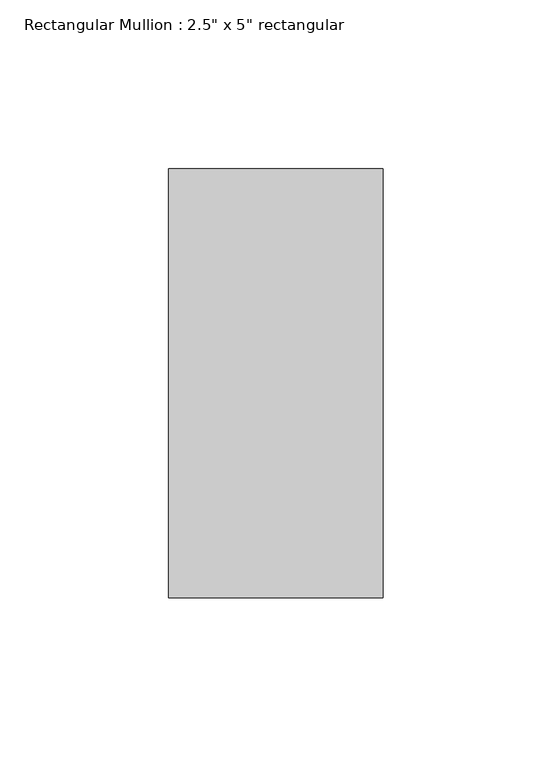
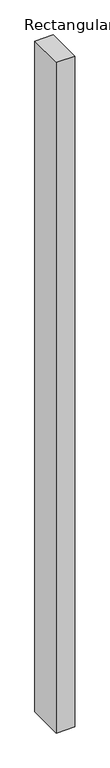
"""IFC4 building model written with IfcOpenShell, lengths in millimetres: member geometry."""

from ifc_helpers import new_model, si_unit, frame, origin, place, context, project, spatial, polyline, outline, extrude, source, transform, mapped, element, save


def member_ee409385(model_context):
    return source(origin(), model_context, "Body", "SweptSolid", [
        extrude(outline(polyline([(0.0, 63.5), (0.0, -63.5), (-63.5, -63.5), (-63.5, 63.5), (0.0, 63.5)])), frame((0.0, 0.0, -2438.4), z_axis=(0.0, 0.0, 1.0), x_axis=(1.0, 0.0, 0.0)), (0.0, 0.0, 1.0), 2438.4),
    ])


if __name__ == "__main__":
    model = new_model("IFC4")
    model_context = context("Model", 3, world=origin())
    ifc_project = project(units=[si_unit("LENGTHUNIT", "METRE", prefix="MILLI")], contexts=[model_context])
    site = spatial("IfcSite", under=ifc_project)
    building = spatial("IfcBuilding", under=site)
    placement = place(None, origin())
    member_shape = member_ee409385(model_context)
    element("IfcMember", 1, ObjectType="Rectangular Mullion : 2.5\" x 5\" rectangular", at=placement, inside=building, context=model_context, shape_type="MappedRepresentation", body=[
        mapped(member_shape, transform((0.0, 0.0, 0.0), x_axis=(1.0, 0.0, 0.0), y_axis=(0.0, 1.0, 0.0), z_axis=(0.0, 0.0, 1.0))),
    ])
    save(model, "model.ifc")

# Revit data of these elements
# Type "Rectangular Mullion : 2.5\" x 5\" rectangular"
#   built-in parameter 1007304 = 0.416667 (stored number, unit not read)
#   built-in parameter 1007301 = 0.104167 (stored number, unit not read)
#   built-in parameter 1007300 = 0.104167 (stored number, unit not read)
# Element 1 (IfcMember, "Rectangular Mullion : 2.5\" x 5\" rectangular")
#   Materials on its faces: "BLACK MATERIAL"
# Materials
#   "BLACK MATERIAL": class "Generic", colour RGB 120 120 120, transparency 0, Cost = 0
